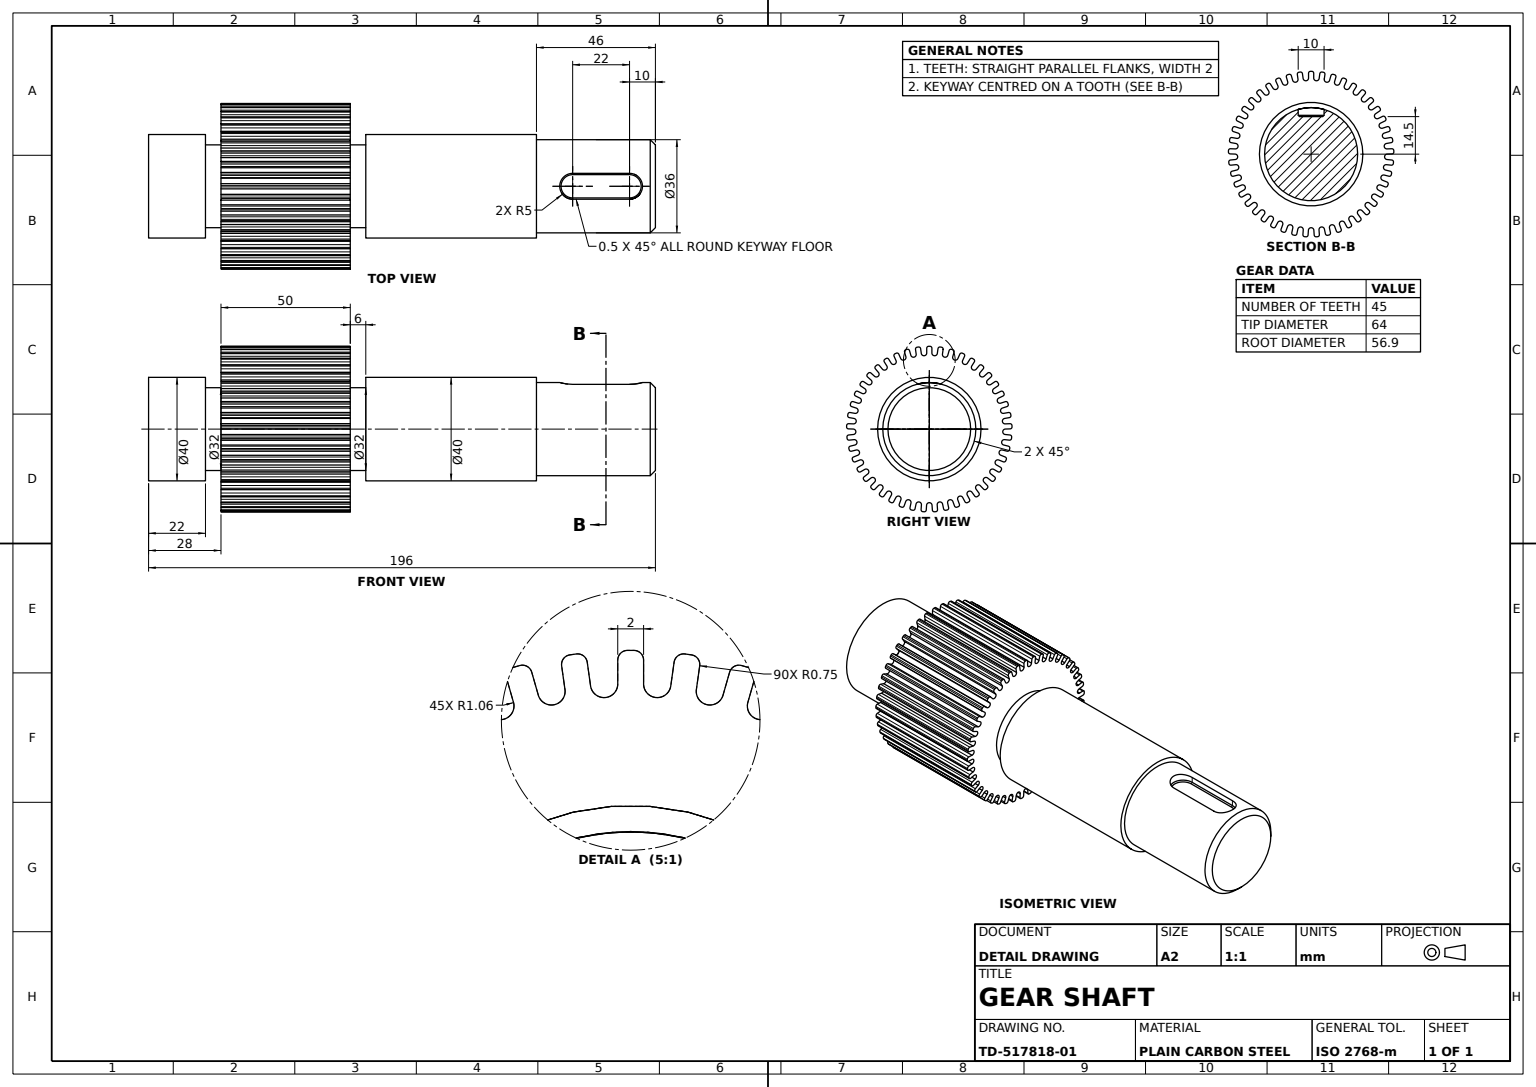
from build123d import *

# Parameters (mm, degrees)
GEAR_TEETH_SKETCH_OUTSIDE_W    = 109.178
GEAR_TEETH_SKETCH_OUTSIDE_H    = 109.178
GEAR_TEETH_CUT_DEPTH           = 50
KEYWAY_CUT_5X22_DEPTH          = 7
SHAFT_EDGE_CHAMFER_2MM_SIZE    = 2
KEYWAY_EDGE_CHAMFER_0_5MM_SIZE = 0.5


with BuildPart() as part:
    # Shaft Profile Sketch → Shaft Body Revolve (revolve)
    with BuildSketch(Plane.XY, mode=Mode.PRIVATE) as shaft_body_revolve_sk:
        Polygon((0, 0), (0, 20), (22, 20), (22, 16), (28, 16), (28, 32), (78, 32), (78, 16), (84, 16), (84, 20), (150, 20), (150, 18), (196, 18), (196, 0), align=None)
    revolve(shaft_body_revolve_sk.sketch.rotate(Axis((196, 0, 0), (-1, 0, 0)), 90), axis=Axis((196, 0, 0), (-1, 0, 0)))

    # Gear Teeth Sketch outside → Gear Teeth Cut (cut)
    with BuildSketch(Plane(origin=(78, 0, 0), x_dir=(0, 0, -1), z_dir=(1, 0, 0))):
        Rectangle(GEAR_TEETH_SKETCH_OUTSIDE_W, GEAR_TEETH_SKETCH_OUTSIDE_H)
        with BuildLine():
            Line((-1, 29.482704379), (-1, 31.248999984))
            ThreePointArc((-1, 31.248999984), (-0.78244718, 31.77720449), (-0.256, 31.998975984))
            ThreePointArc((-0.256, 31.998975984), (0, 32), (0.256, 31.998975984))
            ThreePointArc((0.256, 31.998975984), (0.78244718, 31.77720449), (1, 31.248999984))
            Line((1, 31.248999984), (1, 29.482704379))
            ThreePointArc((1, 29.482704379), (1.982590387, 28.352363441), (3.112931324, 29.334953828))
            Line((3.112931324, 29.334953828), (3.358752161, 31.084059965))
            ThreePointArc((3.358752161, 31.084059965), (3.64769963, 31.576846521), (4.19988809, 31.723192463))
            ThreePointArc((4.19988809, 31.723192463), (4.453539231, 31.6885782), (4.706905341, 31.651935835))
            ThreePointArc((4.706905341, 31.651935835), (5.197364547, 31.35905532), (5.339288298, 30.805713763))
            Line((5.339288298, 30.805713763), (5.093467462, 29.056607626))
            ThreePointArc((5.093467462, 29.056607626), (5.909182293, 27.800516937), (7.165272981, 28.616231768))
            Line((7.165272981, 28.616231768), (7.652130032, 30.314104077))
            ThreePointArc((7.652130032, 30.314104077), (8.006848117, 30.761881152), (8.574030135, 30.829953085))
            ThreePointArc((8.574030135, 30.829953085), (8.820395386, 30.76037427), (9.066196123, 30.688826759))
            ThreePointArc((9.066196123, 30.688826759), (9.511121125, 30.330537808), (9.574653423, 29.762829365))
            Line((9.574653423, 29.762829365), (9.087796373, 28.064957056))
            ThreePointArc((9.087796373, 28.064957056), (9.720758687, 26.707564993), (11.07815075, 27.340527308))
            Line((11.07815075, 27.340527308), (11.796567895, 28.954118634))
            ThreePointArc((11.796567895, 28.954118634), (12.210152413, 29.348170758), (12.781288436, 29.33664374))
            ThreePointArc((12.781288436, 29.33664374), (13.015572578, 29.233454645), (13.249023711, 29.128394578))
            ThreePointArc((13.249023711, 29.128394578), (13.639754548, 28.711670879), (13.623658811, 28.140645348))
            Line((13.623658811, 28.140645348), (12.905241666, 26.527054021))
            ThreePointArc((12.905241666, 26.527054021), (13.343131571, 25.094780677), (14.775404916, 25.532670582))
            Line((14.775404916, 25.532670582), (15.711398983, 27.030574207))
            ThreePointArc((15.711398983, 27.030574207), (16.175799981, 27.363231603), (16.739773497, 27.272329994))
            ThreePointArc((16.739773497, 27.272329994), (16.957416455, 27.137539077), (17.173974122, 27.00101133))
            ThreePointArc((17.173974122, 27.00101133), (17.502905664, 26.533963935), (17.407495176, 25.970735679))
            Line((17.407495176, 25.970735679), (16.471501108, 24.472832054))
            ThreePointArc((16.471501108, 24.472832054), (16.705795577, 22.993554999), (18.185072632, 23.227849467))
            Line((18.185072632, 23.227849467), (19.320425562, 24.5809104))
            ThreePointArc((19.320425562, 24.5809104), (19.826604002, 24.84569827), (20.372437907, 24.677191366))
            ThreePointArc((20.372437907, 24.677191366), (20.56920351, 24.51342218), (20.764652662, 24.34808411))
            ThreePointArc((20.764652662, 24.34808411), (21.025382631, 23.839803564), (20.852514448, 23.295335181))
            Line((20.852514448, 23.295335181), (19.717161518, 21.942274248))
            ThreePointArc((19.717161518, 21.942274248), (19.743300274, 20.444785928), (21.240788594, 20.470924684))
            Line((21.240788594, 20.470924684), (22.553402033, 21.652807133))
            ThreePointArc((22.553402033, 21.652807133), (23.091505728, 21.844571682), (23.608575988, 21.601739278))
            ThreePointArc((23.608575988, 21.601739278), (23.780634415, 21.412179403), (23.951170858, 21.221249127))
            ThreePointArc((23.951170858, 21.221249127), (24.138624441, 20.681628535), (23.891663246, 20.166517482))
            Line((23.891663246, 20.166517482), (22.579049807, 18.984635033))
            ThreePointArc((22.579049807, 18.984635033), (22.396524089, 17.498082354), (23.883076767, 17.315556636))
            Line((23.883076767, 17.315556636), (25.347402188, 18.303256604))
            ThreePointArc((25.347402188, 18.303256604), (25.906957562, 18.418265354), (26.38519999, 18.105833907))
            ThreePointArc((26.38519999, 18.105833907), (26.529202322, 17.894172911), (26.671506757, 17.68136667))
            ThreePointArc((26.671506757, 17.68136667), (26.782035384, 17.120909132), (26.465787995, 16.645181459))
            Line((26.465787995, 16.645181459), (25.001462574, 15.657481491))
            ThreePointArc((25.001462574, 15.657481491), (24.613825038, 14.210798511), (26.060508018, 13.823160975))
            Line((26.060508018, 13.823160975), (27.648043992, 14.597454005))
            ThreePointArc((27.648043992, 14.597454005), (28.218159936, 14.633468441), (28.648266088, 14.257519074))
            ThreePointArc((28.648266088, 14.257519074), (28.761409482, 14.027876697), (28.872712115, 13.797336522))
            ThreePointArc((28.872712115, 13.797336522), (28.904164471, 13.226950707), (28.524786285, 12.799865913))
            Line((28.524786285, 12.799865913), (26.937250311, 12.025572883))
            ThreePointArc((26.937250311, 12.025572883), (26.352045881, 10.64691764), (27.730701123, 10.06171321))
            Line((27.730701123, 10.06171321), (29.410548068, 10.607528569))
            ThreePointArc((29.410548068, 10.607528569), (29.980127924, 10.563847711), (30.353726273, 10.13169785))
            ThreePointArc((30.353726273, 10.13169785), (30.433808521, 9.88854382), (30.511942975, 9.644756913))
            ThreePointArc((30.511942975, 9.644756913), (30.463706876, 9.075544731), (30.028582057, 8.705415536))
            Line((30.028582057, 8.705415536), (28.348735112, 8.159600177))
            ThreePointArc((28.348735112, 8.159600177), (27.577354125, 6.875806628), (28.861147675, 6.104425641))
            Line((28.861147675, 6.104425641), (30.60060928, 6.411139654))
            ThreePointArc((30.60060928, 6.411139654), (31.158566824, 6.288613701), (31.468385704, 5.808674652))
            ThreePointArc((31.468385704, 5.808674652), (31.513848096, 5.556741685), (31.557293571, 5.304453082))
            ThreePointArc((31.557293571, 5.304453082), (31.430307878, 4.747493601), (30.947905636, 4.441524148))
            Line((30.947905636, 4.441524148), (29.20844403, 4.134810135))
            ThreePointArc((29.20844403, 4.134810135), (28.265900541, 2.97086586), (29.429844815, 2.028322371))
            Line((29.429844815, 2.028322371), (31.195064441, 2.089965199))
            ThreePointArc((31.195064441, 2.089965199), (31.730539663, 1.890978978), (31.970548801, 1.372592209))
            ThreePointArc((31.970548801, 1.372592209), (31.980506465, 1.116783894), (31.988417343, 0.860904105))
            ThreePointArc((31.988417343, 0.860904105), (31.785153688, 0.327037909), (31.264863434, 0.091183545))
            Line((31.264863434, 0.091183545), (29.499643809, 0.029540717))
            ThreePointArc((29.499643809, 0.029540717), (28.404283354, -0.991899432), (29.425723503, -2.087259886))
            Line((29.425723503, -2.087259886), (31.182343156, -2.271888052))
            ThreePointArc((31.182343156, -2.271888052), (31.68491364, -2.543461499), (31.850441532, -3.09020618))
            ThreePointArc((31.850441532, -3.09020618), (31.824700652, -3.344910825), (31.796922958, -3.599401391))
            ThreePointArc((31.796922958, -3.599401391), (31.521337637, -4.099783205), (30.973286229, -4.260931842))
            Line((30.973286229, -4.260931842), (29.216666576, -4.076303677))
            ThreePointArc((29.216666576, -4.076303677), (27.989809101, -4.935358529), (28.848863954, -6.162216004))
            Line((28.848863954, -6.162216004), (30.56269303, -6.589521585))
            ThreePointArc((30.56269303, -6.589521585), (31.022576815, -6.928396392), (31.110401647, -7.492857221))
            ThreePointArc((31.110401647, -7.492857221), (31.049463241, -7.741500659), (30.986537637, -7.989648633))
            ThreePointArc((30.986537637, -7.989648633), (30.643994604, -8.446806702), (30.078849239, -8.530113038))
            Line((30.078849239, -8.530113038), (28.365020162, -8.102807457))
            ThreePointArc((28.365020162, -8.102807457), (27.030545052, -8.782756487), (27.710494083, -10.117231598))
            Line((27.710494083, -10.117231598), (29.34817485, -10.778897577))
            ThreePointArc((29.34817485, -10.778897577), (29.756420819, -11.178477929), (29.764833183, -11.749668319))
            ThreePointArc((29.764833183, -11.749668319), (29.669883346, -11.987410989), (29.573034607, -12.224386453))
            ThreePointArc((29.573034607, -12.224386453), (29.170201073, -12.629422715), (28.598961663, -12.633265286))
            Line((28.598961663, -12.633265286), (26.961280896, -11.971599307))
            ThreePointArc((26.961280896, -11.971599307), (25.545162191, -12.459208081), (26.032770964, -13.875326786))
            Line((26.032770964, -13.875326786), (27.562427829, -14.758474588))
            ThreePointArc((27.562427829, -14.758474588), (27.91108994, -15.21098311), (27.839926097, -15.777785488))
            ThreePointArc((27.839926097, -15.777785488), (27.712812921, -16), (27.583926097, -16.221190495))
            ThreePointArc((27.583926097, -16.221190495), (27.128642759, -16.56622138), (26.562427829, -16.490525396))
            Line((26.562427829, -16.490525396), (25.032770964, -15.607377593))
            ThreePointArc((25.032770964, -15.607377593), (23.562571804, -15.893155361), (23.848349571, -17.363354521))
            Line((23.848349571, -17.363354521), (25.240209502, -18.450794679))
            ThreePointArc((25.240209502, -18.450794679), (25.522501443, -18.947423806), (25.373146517, -19.49880601))
            ThreePointArc((25.373146517, -19.49880601), (25.216344115, -19.70116721), (25.057927842, -19.902267516))
            ThreePointArc((25.057927842, -19.902267516), (24.559056272, -20.18057739), (24.008886552, -20.026816186))
            Line((24.008886552, -20.026816186), (22.617026621, -18.939376028))
            ThreePointArc((22.617026621, -18.939376028), (21.121362759, -19.01776045), (21.199747181, -20.513424311))
            Line((21.199747181, -20.513424311), (22.426719208, -21.783991039))
            ThreePointArc((22.426719208, -21.783991039), (22.637146487, -22.31507445), (22.412507502, -22.840304452))
            ThreePointArc((22.412507502, -22.840304452), (22.229067855, -23.018873611), (22.044205524, -23.195969538))
            ThreePointArc((22.044205524, -23.195969538), (21.51145569, -23.402141416), (20.988039607, -23.17330778))
            Line((20.988039607, -23.17330778), (19.76106758, -21.902741052))
            ThreePointArc((19.76106758, -21.902741052), (18.269050414, -21.772206464), (18.138515826, -23.26422363))
            Line((18.138515826, -23.26422363), (19.176718334, -24.693186792))
            ThreePointArc((19.176718334, -24.693186792), (19.311185224, -25.248387553), (19.015634522, -25.737242349))
            ThreePointArc((19.015634522, -25.737242349), (18.809128073, -25.88854382), (18.601417821, -26.038188398))
            ThreePointArc((18.601417821, -26.038188398), (18.045159092, -26.168209379), (17.558684345, -25.868757297))
            Line((17.558684345, -25.868757297), (16.520481837, -24.439794135))
            ThreePointArc((16.520481837, -24.439794135), (15.061151783, -24.102881245), (14.724238893, -25.5622113))
            Line((14.724238893, -25.5622113), (15.553464451, -27.121757752))
            ThreePointArc((15.553464451, -27.121757752), (15.609353707, -27.690269511), (15.248643846, -28.133234099))
            ThreePointArc((15.248643846, -28.133234099), (15.023090009, -28.254322971), (14.796574679, -28.373603539))
            ThreePointArc((14.796574679, -28.373603539), (14.227633998, -28.424942913), (13.787569265, -28.060700878))
            Line((13.787569265, -28.060700878), (12.958343707, -26.501154425))
            ThreePointArc((12.958343707, -26.501154425), (11.560104964, -25.964420859), (11.023371398, -27.362659602))
            Line((11.023371398, -27.362659602), (11.627480074, -29.022434549))
            ThreePointArc((11.627480074, -29.022434549), (11.603703876, -29.593191872), (11.184855663, -29.981644448))
            ThreePointArc((11.184855663, -29.981644448), (10.944644586, -30.070163865), (10.703733041, -30.156758761))
            ThreePointArc((10.703733041, -30.156758761), (10.133184192, -30.128417265), (9.748094833, -29.706474835))
            Line((9.748094833, -29.706474835), (9.143986157, -28.046699889))
            ThreePointArc((9.143986157, -28.046699889), (7.834053852, -27.320592556), (7.107946518, -28.630524861))
            Line((7.107946518, -28.630524861), (7.475180024, -30.358222669))
            ThreePointArc((7.475180024, -30.358222669), (7.372201147, -30.920116414), (6.903366987, -31.246496191))
            ThreePointArc((6.903366987, -31.246496191), (6.653174106, -31.300723223), (6.402555415, -31.352946977))
            ThreePointArc((6.402555415, -31.352946977), (5.841503483, -31.245476246), (5.518884822, -30.77404605))
            Line((5.518884822, -30.77404605), (5.151651317, -29.046348242))
            ThreePointArc((5.151651317, -29.046348242), (3.955521792, -28.144999995), (3.054173544, -29.341129519))
            Line((3.054173544, -29.341129519), (3.177384097, -31.103122517))
            ThreePointArc((3.177384097, -31.103122517), (2.997206909, -31.645216061), (2.487512125, -31.903170429))
            ThreePointArc((2.487512125, -31.903170429), (2.23220716, -31.922049608), (1.976759331, -31.938885744))
            ThreePointArc((1.976759331, -31.938885744), (1.436124552, -31.754377573), (1.182255997, -31.242635464))
            Line((1.182255997, -31.242635464), (1.059045444, -29.480642467))
            ThreePointArc((1.059045444, -29.480642467), (0, -28.421597023), (-1.059045444, -29.480642467))
            Line((-1.059045444, -29.480642467), (-1.182255997, -31.242635464))
            ThreePointArc((-1.182255997, -31.242635464), (-1.436124552, -31.754377573), (-1.976759331, -31.938885744))
            ThreePointArc((-1.976759331, -31.938885744), (-2.23220716, -31.922049608), (-2.487512125, -31.903170429))
            ThreePointArc((-2.487512125, -31.903170429), (-2.997206909, -31.645216061), (-3.177384097, -31.103122517))
            Line((-3.177384097, -31.103122517), (-3.054173544, -29.341129519))
            ThreePointArc((-3.054173544, -29.341129519), (-3.955521792, -28.144999995), (-5.151651317, -29.046348242))
            Line((-5.151651317, -29.046348242), (-5.518884822, -30.77404605))
            ThreePointArc((-5.518884822, -30.77404605), (-5.841503483, -31.245476246), (-6.402555415, -31.352946977))
            ThreePointArc((-6.402555415, -31.352946977), (-6.653174106, -31.300723223), (-6.903366987, -31.246496191))
            ThreePointArc((-6.903366987, -31.246496191), (-7.372201147, -30.920116414), (-7.475180024, -30.358222669))
            Line((-7.475180024, -30.358222669), (-7.107946518, -28.630524861))
            ThreePointArc((-7.107946518, -28.630524861), (-7.834053852, -27.320592556), (-9.143986157, -28.046699889))
            Line((-9.143986157, -28.046699889), (-9.748094833, -29.706474835))
            ThreePointArc((-9.748094833, -29.706474835), (-10.133184192, -30.128417265), (-10.703733041, -30.156758761))
            ThreePointArc((-10.703733041, -30.156758761), (-10.944644586, -30.070163865), (-11.184855663, -29.981644448))
            ThreePointArc((-11.184855663, -29.981644448), (-11.603703876, -29.593191872), (-11.627480074, -29.022434549))
            Line((-11.627480074, -29.022434549), (-11.023371398, -27.362659602))
            ThreePointArc((-11.023371398, -27.362659602), (-11.560104964, -25.964420859), (-12.958343707, -26.501154425))
            Line((-12.958343707, -26.501154425), (-13.787569265, -28.060700878))
            ThreePointArc((-13.787569265, -28.060700878), (-14.227633998, -28.424942913), (-14.796574679, -28.373603539))
            ThreePointArc((-14.796574679, -28.373603539), (-15.023090009, -28.254322971), (-15.248643846, -28.133234099))
            ThreePointArc((-15.248643846, -28.133234099), (-15.609353707, -27.690269511), (-15.553464451, -27.121757752))
            Line((-15.553464451, -27.121757752), (-14.724238893, -25.5622113))
            ThreePointArc((-14.724238893, -25.5622113), (-15.061151783, -24.102881245), (-16.520481837, -24.439794135))
            Line((-16.520481837, -24.439794135), (-17.558684345, -25.868757297))
            ThreePointArc((-17.558684345, -25.868757297), (-18.045159092, -26.168209379), (-18.601417821, -26.038188398))
            ThreePointArc((-18.601417821, -26.038188398), (-18.809128073, -25.88854382), (-19.015634522, -25.737242349))
            ThreePointArc((-19.015634522, -25.737242349), (-19.311185224, -25.248387553), (-19.176718334, -24.693186792))
            Line((-19.176718334, -24.693186792), (-18.138515826, -23.26422363))
            ThreePointArc((-18.138515826, -23.26422363), (-18.269050414, -21.772206464), (-19.76106758, -21.902741052))
            Line((-19.76106758, -21.902741052), (-20.988039607, -23.17330778))
            ThreePointArc((-20.988039607, -23.17330778), (-21.51145569, -23.402141416), (-22.044205524, -23.195969538))
            ThreePointArc((-22.044205524, -23.195969538), (-22.229067855, -23.018873611), (-22.412507502, -22.840304452))
            ThreePointArc((-22.412507502, -22.840304452), (-22.637146487, -22.31507445), (-22.426719208, -21.783991039))
            Line((-22.426719208, -21.783991039), (-21.199747181, -20.513424311))
            ThreePointArc((-21.199747181, -20.513424311), (-21.121362759, -19.01776045), (-22.617026621, -18.939376028))
            Line((-22.617026621, -18.939376028), (-24.008886552, -20.026816186))
            ThreePointArc((-24.008886552, -20.026816186), (-24.559056272, -20.18057739), (-25.057927842, -19.902267516))
            ThreePointArc((-25.057927842, -19.902267516), (-25.216344115, -19.70116721), (-25.373146517, -19.49880601))
            ThreePointArc((-25.373146517, -19.49880601), (-25.522501443, -18.947423806), (-25.240209502, -18.450794679))
            Line((-25.240209502, -18.450794679), (-23.848349571, -17.363354521))
            ThreePointArc((-23.848349571, -17.363354521), (-23.562571804, -15.893155361), (-25.032770964, -15.607377593))
            Line((-25.032770964, -15.607377593), (-26.562427829, -16.490525396))
            ThreePointArc((-26.562427829, -16.490525396), (-27.128642759, -16.56622138), (-27.583926097, -16.221190495))
            ThreePointArc((-27.583926097, -16.221190495), (-27.712812921, -16), (-27.839926097, -15.777785488))
            ThreePointArc((-27.839926097, -15.777785488), (-27.91108994, -15.21098311), (-27.562427829, -14.758474588))
            Line((-27.562427829, -14.758474588), (-26.032770964, -13.875326786))
            ThreePointArc((-26.032770964, -13.875326786), (-25.545162191, -12.459208081), (-26.961280896, -11.971599307))
            Line((-26.961280896, -11.971599307), (-28.598961663, -12.633265286))
            ThreePointArc((-28.598961663, -12.633265286), (-29.170201073, -12.629422715), (-29.573034607, -12.224386453))
            ThreePointArc((-29.573034607, -12.224386453), (-29.669883346, -11.987410989), (-29.764833183, -11.749668319))
            ThreePointArc((-29.764833183, -11.749668319), (-29.756420819, -11.178477929), (-29.34817485, -10.778897577))
            Line((-29.34817485, -10.778897577), (-27.710494083, -10.117231598))
            ThreePointArc((-27.710494083, -10.117231598), (-27.030545052, -8.782756487), (-28.365020162, -8.102807457))
            Line((-28.365020162, -8.102807457), (-30.078849239, -8.530113038))
            ThreePointArc((-30.078849239, -8.530113038), (-30.643994604, -8.446806702), (-30.986537637, -7.989648633))
            ThreePointArc((-30.986537637, -7.989648633), (-31.049463241, -7.741500659), (-31.110401647, -7.492857221))
            ThreePointArc((-31.110401647, -7.492857221), (-31.022576815, -6.928396392), (-30.56269303, -6.589521585))
            Line((-30.56269303, -6.589521585), (-28.848863954, -6.162216004))
            ThreePointArc((-28.848863954, -6.162216004), (-27.989809101, -4.935358529), (-29.216666576, -4.076303677))
            Line((-29.216666576, -4.076303677), (-30.973286229, -4.260931842))
            ThreePointArc((-30.973286229, -4.260931842), (-31.521337637, -4.099783205), (-31.796922958, -3.599401391))
            ThreePointArc((-31.796922958, -3.599401391), (-31.824700652, -3.344910825), (-31.850441532, -3.09020618))
            ThreePointArc((-31.850441532, -3.09020618), (-31.68491364, -2.543461499), (-31.182343156, -2.271888052))
            Line((-31.182343156, -2.271888052), (-29.425723503, -2.087259886))
            ThreePointArc((-29.425723503, -2.087259886), (-28.404283354, -0.991899432), (-29.499643809, 0.029540717))
            Line((-29.499643809, 0.029540717), (-31.264863434, 0.091183545))
            ThreePointArc((-31.264863434, 0.091183545), (-31.785153688, 0.327037909), (-31.988417343, 0.860904105))
            ThreePointArc((-31.988417343, 0.860904105), (-31.980506465, 1.116783894), (-31.970548801, 1.372592209))
            ThreePointArc((-31.970548801, 1.372592209), (-31.730539663, 1.890978978), (-31.195064441, 2.089965199))
            Line((-31.195064441, 2.089965199), (-29.429844815, 2.028322371))
            ThreePointArc((-29.429844815, 2.028322371), (-28.265900541, 2.97086586), (-29.20844403, 4.134810135))
            Line((-29.20844403, 4.134810135), (-30.947905636, 4.441524148))
            ThreePointArc((-30.947905636, 4.441524148), (-31.430307878, 4.747493601), (-31.557293571, 5.304453082))
            ThreePointArc((-31.557293571, 5.304453082), (-31.513848096, 5.556741685), (-31.468385704, 5.808674652))
            ThreePointArc((-31.468385704, 5.808674652), (-31.158566824, 6.288613701), (-30.60060928, 6.411139654))
            Line((-30.60060928, 6.411139654), (-28.861147675, 6.104425641))
            ThreePointArc((-28.861147675, 6.104425641), (-27.577354125, 6.875806628), (-28.348735112, 8.159600177))
            Line((-28.348735112, 8.159600177), (-30.028582057, 8.705415536))
            ThreePointArc((-30.028582057, 8.705415536), (-30.463706876, 9.075544731), (-30.511942975, 9.644756913))
            ThreePointArc((-30.511942975, 9.644756913), (-30.433808521, 9.88854382), (-30.353726273, 10.13169785))
            ThreePointArc((-30.353726273, 10.13169785), (-29.980127924, 10.563847711), (-29.410548068, 10.607528569))
            Line((-29.410548068, 10.607528569), (-27.730701123, 10.06171321))
            ThreePointArc((-27.730701123, 10.06171321), (-26.352045881, 10.64691764), (-26.937250311, 12.025572883))
            Line((-26.937250311, 12.025572883), (-28.524786285, 12.799865913))
            ThreePointArc((-28.524786285, 12.799865913), (-28.904164471, 13.226950707), (-28.872712115, 13.797336522))
            ThreePointArc((-28.872712115, 13.797336522), (-28.761409482, 14.027876697), (-28.648266088, 14.257519074))
            ThreePointArc((-28.648266088, 14.257519074), (-28.218159936, 14.633468441), (-27.648043992, 14.597454005))
            Line((-27.648043992, 14.597454005), (-26.060508018, 13.823160975))
            ThreePointArc((-26.060508018, 13.823160975), (-24.613825038, 14.210798511), (-25.001462574, 15.657481491))
            Line((-25.001462574, 15.657481491), (-26.465787995, 16.645181459))
            ThreePointArc((-26.465787995, 16.645181459), (-26.782035384, 17.120909132), (-26.671506757, 17.68136667))
            ThreePointArc((-26.671506757, 17.68136667), (-26.529202322, 17.894172911), (-26.38519999, 18.105833907))
            ThreePointArc((-26.38519999, 18.105833907), (-25.906957562, 18.418265354), (-25.347402188, 18.303256604))
            Line((-25.347402188, 18.303256604), (-23.883076767, 17.315556636))
            ThreePointArc((-23.883076767, 17.315556636), (-22.396524089, 17.498082354), (-22.579049807, 18.984635033))
            Line((-22.579049807, 18.984635033), (-23.891663246, 20.166517482))
            ThreePointArc((-23.891663246, 20.166517482), (-24.138624441, 20.681628535), (-23.951170858, 21.221249127))
            ThreePointArc((-23.951170858, 21.221249127), (-23.780634415, 21.412179403), (-23.608575988, 21.601739278))
            ThreePointArc((-23.608575988, 21.601739278), (-23.091505728, 21.844571682), (-22.553402033, 21.652807133))
            Line((-22.553402033, 21.652807133), (-21.240788594, 20.470924684))
            ThreePointArc((-21.240788594, 20.470924684), (-19.743300274, 20.444785928), (-19.717161518, 21.942274248))
            Line((-19.717161518, 21.942274248), (-20.852514448, 23.295335181))
            ThreePointArc((-20.852514448, 23.295335181), (-21.025382631, 23.839803564), (-20.764652662, 24.34808411))
            ThreePointArc((-20.764652662, 24.34808411), (-20.56920351, 24.51342218), (-20.372437907, 24.677191366))
            ThreePointArc((-20.372437907, 24.677191366), (-19.826604002, 24.84569827), (-19.320425562, 24.5809104))
            Line((-19.320425562, 24.5809104), (-18.185072632, 23.227849467))
            ThreePointArc((-18.185072632, 23.227849467), (-16.705795577, 22.993554999), (-16.471501108, 24.472832054))
            Line((-16.471501108, 24.472832054), (-17.407495176, 25.970735679))
            ThreePointArc((-17.407495176, 25.970735679), (-17.502905664, 26.533963935), (-17.173974122, 27.00101133))
            ThreePointArc((-17.173974122, 27.00101133), (-16.957416455, 27.137539077), (-16.739773497, 27.272329994))
            ThreePointArc((-16.739773497, 27.272329994), (-16.175799981, 27.363231603), (-15.711398983, 27.030574207))
            Line((-15.711398983, 27.030574207), (-14.775404916, 25.532670582))
            ThreePointArc((-14.775404916, 25.532670582), (-13.343131571, 25.094780677), (-12.905241666, 26.527054021))
            Line((-12.905241666, 26.527054021), (-13.623658811, 28.140645348))
            ThreePointArc((-13.623658811, 28.140645348), (-13.639754548, 28.711670879), (-13.249023711, 29.128394578))
            ThreePointArc((-13.249023711, 29.128394578), (-13.015572578, 29.233454645), (-12.781288436, 29.33664374))
            ThreePointArc((-12.781288436, 29.33664374), (-12.210152413, 29.348170758), (-11.796567895, 28.954118634))
            Line((-11.796567895, 28.954118634), (-11.07815075, 27.340527308))
            ThreePointArc((-11.07815075, 27.340527308), (-9.720758687, 26.707564993), (-9.087796373, 28.064957056))
            Line((-9.087796373, 28.064957056), (-9.574653423, 29.762829365))
            ThreePointArc((-9.574653423, 29.762829365), (-9.511121125, 30.330537808), (-9.066196123, 30.688826759))
            ThreePointArc((-9.066196123, 30.688826759), (-8.820395386, 30.76037427), (-8.574030135, 30.829953085))
            ThreePointArc((-8.574030135, 30.829953085), (-8.006848117, 30.761881152), (-7.652130032, 30.314104077))
            Line((-7.652130032, 30.314104077), (-7.165272981, 28.616231768))
            ThreePointArc((-7.165272981, 28.616231768), (-5.909182293, 27.800516937), (-5.093467462, 29.056607626))
            Line((-5.093467462, 29.056607626), (-5.339288298, 30.805713763))
            ThreePointArc((-5.339288298, 30.805713763), (-5.197364547, 31.35905532), (-4.706905341, 31.651935835))
            ThreePointArc((-4.706905341, 31.651935835), (-4.453539231, 31.6885782), (-4.19988809, 31.723192463))
            ThreePointArc((-4.19988809, 31.723192463), (-3.64769963, 31.576846521), (-3.358752161, 31.084059965))
            Line((-3.358752161, 31.084059965), (-3.112931324, 29.334953828))
            ThreePointArc((-3.112931324, 29.334953828), (-1.982590387, 28.352363441), (-1, 29.482704379))
        make_face(mode=Mode.SUBTRACT)
    extrude(amount=-GEAR_TEETH_CUT_DEPTH, mode=Mode.SUBTRACT)

    # Keyway Sketch → Keyway Cut 5x22 (cut)
    with BuildSketch(Plane(origin=(0, 14.5, 0), x_dir=(1, 0, 0), z_dir=(0, 1, 0))):
        with BuildLine():
            Line((164, 5), (186, 5))
            ThreePointArc((186, 5), (191, 0), (186, -5))
            Line((186, -5), (164, -5))
            ThreePointArc((164, -5), (159, 0), (164, 5))
        make_face()
    extrude(amount=KEYWAY_CUT_5X22_DEPTH, mode=Mode.SUBTRACT)

    # Shaft Edge Chamfer 2mm
    shaft_edge_chamfer_2mm_edges = [part.edges().sort_by_distance(p)[0] for p in [
        (196, 0, 18),
    ]]
    chamfer(shaft_edge_chamfer_2mm_edges, length=SHAFT_EDGE_CHAMFER_2MM_SIZE)

    # Keyway Edge Chamfer 0.5mm
    keyway_edge_chamfer_0_5mm_edges = [part.edges().sort_by_distance(p)[0] for p in [
        (159, 14.5, 0),
        (175, 14.5, 5),
        (191, 14.5, 0),
        (175, 14.5, -5),
    ]]
    chamfer(keyway_edge_chamfer_0_5mm_edges, length=KEYWAY_EDGE_CHAMFER_0_5MM_SIZE)


solid = part.part
